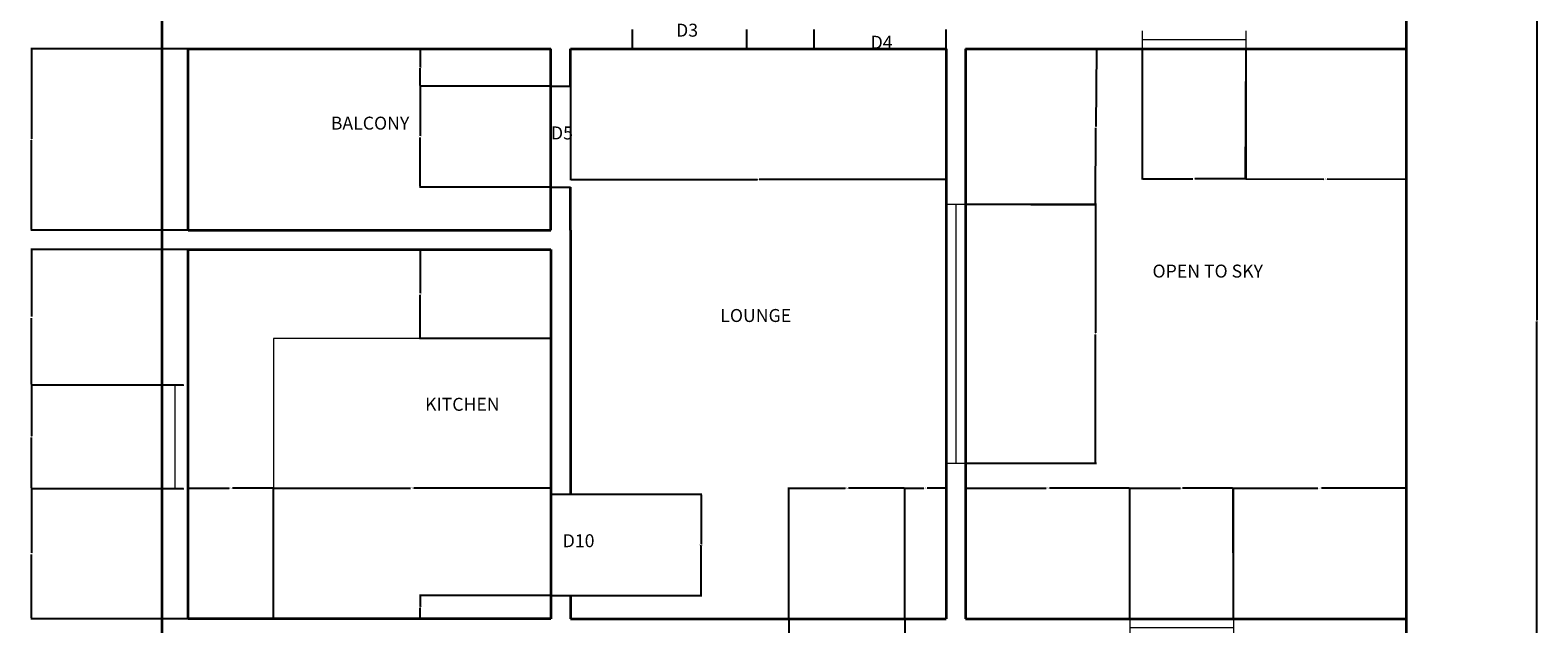
# Model space of a CAD drawing. Units: inches. Extents: x 301 to 1174, y -458 to 167.
# Tile 3 of 4: x 825 to 1174, y -203 to -66. Entities that reach past the tile are written whole.
import ezdxf

# ---------------------------------------------------------------- set-up
doc = ezdxf.new("R2010")
doc.units = ezdxf.units.IN
doc.header["$MEASUREMENT"] = 0
for name, color, linetype, lineweight in [('A-ANNO-DIMS', 2, 'Continuous', 18), ('A-ANNO-TEXT', 7, 'Continuous', 25), ('A-AREA-IDEN', 7, 'Continuous', 18), ('A-DOOR', 3, 'Continuous', 25), ('A-FLOR-FIXT', 8, 'Continuous', 18), ('A-GLAZ', 4, 'Continuous', 18), ('A-WALL', 7, 'Continuous', 35)]:
    doc.layers.add(name, color=color, linetype=linetype, lineweight=lineweight)
doc.styles.get("Standard").update_dxf_attribs({"font": 'arial.ttf'})
doc.dimstyles.get("Standard").update_dxf_attribs({"dimtxt": 0.18, "dimasz": 0.18, "dimexe": 0.18, "dimexo": 0.0625, "dimgap": 0.09, "dimtad": 0, "dimtih": 1, "dimtoh": 1, "dimdec": 4, "dimzin": 0, "dimdsep": 46, "dimtxsty": 'Standard', "dimcen": 0.09, "dimadec": 0, "dimazin": 0, "dimtfac": 1, "dimtdec": 4, "dimtofl": 0, "dimtmove": 0, "dimatfit": 3, "dimfxl": 1, "dimtolj": 1, "dimtzin": 0, "dimarcsym": 0})

# ---------------------------------------------------------------- blocks, each defined once
blk = doc.blocks.new('*U2')
for p, q in [((0, 4), (0, 0)), ((24, 4), (24, 0)), ((0, 2), (24, 2))]:
    blk.add_line(p, q)
blk = doc.blocks.new('*U4')
for p, q in [((0, 4), (0, 0)), ((60, 4), (60, 0)), ((0, 2), (60, 2))]:
    blk.add_line(p, q)
blk = doc.blocks.new('*D39')
at = {"layer": 'A-ANNO-DIMS', "color": 0, "lineweight": -2, "transparency": 16777216}
for p, q in [((1143.26, 136.8), (1173.63, 136.8)), ((1173.45, 136.62), (1173.45, -133.02)), ((1173.45, -403.02), (1173.45, -133.38)), ((1143.26, -403.2), (1173.63, -403.2))]:
    blk.add_line(p, q, dxfattribs=at)
at = {"layer": 'A-ANNO-DIMS', "color": 0, "transparency": 16777216}
for points in [[(1173.42, 136.62), (1173.48, 136.62), (1173.45, 136.8)], [(1173.42, -403.02), (1173.48, -403.02), (1173.45, -403.2)]]:
    blk.add_solid(points, dxfattribs=at)
at = {"layer": 'Defpoints', "color": 0, "transparency": 16777216}
for p in [(1143.2, 136.8), (1173.45, 136.8), (1143.2, -403.2)]:
    blk.add_point(p, dxfattribs=at)
at = {"layer": 'A-ANNO-DIMS', "color": 0, "transparency": 16777216, "insert": (1173.45, -133.2), "char_height": 0.18, "attachment_point": 5}
blk.add_mtext('\\A1;540', dxfattribs=at)
blk = doc.blocks.new('*D49')
at = {"layer": 'A-ANNO-DIMS', "color": 0, "lineweight": -2, "transparency": 16777216}
for p, q in [((861.2, -202.14), (861.2, -171.77)), ((861.38, -171.95), (870.71, -171.95)), ((880.81, -171.95), (871.48, -171.95)), ((880.99, -202.14), (880.99, -171.77))]:
    blk.add_line(p, q, dxfattribs=at)
at = {"layer": 'A-ANNO-DIMS', "color": 0, "transparency": 16777216}
for points in [[(861.38, -171.92), (861.38, -171.98), (861.2, -171.95)], [(880.81, -171.92), (880.81, -171.98), (880.99, -171.95)]]:
    blk.add_solid(points, dxfattribs=at)
at = {"layer": 'Defpoints', "color": 0, "transparency": 16777216}
for p in [(880.99, -171.95), (861.2, -202.2), (880.99, -202.2)]:
    blk.add_point(p, dxfattribs=at)
at = {"layer": 'A-ANNO-DIMS', "color": 0, "transparency": 16777216, "insert": (871.09, -171.95), "char_height": 0.18, "attachment_point": 5}
blk.add_mtext('\\A1;19.79', dxfattribs=at)
blk = doc.blocks.new('*D50')
at = {"layer": 'A-ANNO-DIMS', "color": 0, "lineweight": -2, "transparency": 16777216}
for p, q in [((880.99, -202.14), (880.99, -171.77)), ((881.17, -171.95), (912.72, -171.95)), ((945.02, -171.95), (913.47, -171.95)), ((945.2, -202.14), (945.2, -171.77))]:
    blk.add_line(p, q, dxfattribs=at)
at = {"layer": 'A-ANNO-DIMS', "color": 0, "transparency": 16777216}
for points in [[(881.17, -171.92), (881.17, -171.98), (880.99, -171.95)], [(945.02, -171.92), (945.02, -171.98), (945.2, -171.95)]]:
    blk.add_solid(points, dxfattribs=at)
at = {"layer": 'Defpoints', "color": 0, "transparency": 16777216}
for p in [(945.2, -171.95), (880.99, -202.2), (945.2, -202.2)]:
    blk.add_point(p, dxfattribs=at)
at = {"layer": 'A-ANNO-DIMS', "color": 0, "transparency": 16777216, "insert": (913.09, -171.95), "char_height": 0.18, "attachment_point": 5}
blk.add_mtext('\\A1;64.21', dxfattribs=at)
blk = doc.blocks.new('*D51')
at = {"layer": 'A-ANNO-DIMS', "color": 0, "lineweight": -2, "transparency": 16777216}
for p, q in [((945.13, -116.7), (914.77, -116.7)), ((914.95, -116.88), (914.95, -126.82)), ((914.95, -137.13), (914.95, -127.18)), ((945.13, -137.31), (914.77, -137.31))]:
    blk.add_line(p, q, dxfattribs=at)
at = {"layer": 'A-ANNO-DIMS', "color": 0, "transparency": 16777216}
for points in [[(914.92, -116.88), (914.98, -116.88), (914.95, -116.7)], [(914.92, -137.13), (914.98, -137.13), (914.95, -137.31)]]:
    blk.add_solid(points, dxfattribs=at)
at = {"layer": 'Defpoints', "color": 0, "transparency": 16777216}
for p in [(914.95, -116.7), (945.2, -116.7), (945.2, -137.31)]:
    blk.add_point(p, dxfattribs=at)
at = {"layer": 'A-ANNO-DIMS', "color": 0, "transparency": 16777216, "insert": (914.95, -127), "char_height": 0.18, "attachment_point": 5}
blk.add_mtext('\\A1;20.608', dxfattribs=at)
blk = doc.blocks.new('*D52')
at = {"layer": 'A-ANNO-DIMS', "color": 0, "lineweight": -2, "transparency": 16777216}
for p, q in [((949.7, -70.26), (949.7, -100.63)), ((1036.7, -70.26), (1036.7, -100.63)), ((949.88, -100.45), (992.98, -100.45)), ((1036.52, -100.45), (993.42, -100.45))]:
    blk.add_line(p, q, dxfattribs=at)
at = {"layer": 'A-ANNO-DIMS', "color": 0, "transparency": 16777216}
for points in [[(949.88, -100.42), (949.88, -100.48), (949.7, -100.45)], [(1036.52, -100.42), (1036.52, -100.48), (1036.7, -100.45)]]:
    blk.add_solid(points, dxfattribs=at)
at = {"layer": 'Defpoints', "color": 0, "transparency": 16777216}
for p in [(949.7, -70.2), (1036.7, -70.2), (949.7, -100.45)]:
    blk.add_point(p, dxfattribs=at)
at = {"layer": 'A-ANNO-DIMS', "color": 0, "transparency": 16777216, "insert": (993.2, -100.45), "char_height": 0.18, "attachment_point": 5}
blk.add_mtext('\\A1;87', dxfattribs=at)
blk = doc.blocks.new('*D59')
at = {"layer": 'A-ANNO-DIMS', "color": 0, "lineweight": -2, "transparency": 16777216}
for p, q in [((861.13, -70.2), (824.77, -70.2)), ((824.95, -70.38), (824.95, -91.02)), ((824.95, -112.02), (824.95, -91.38)), ((861.13, -112.2), (824.77, -112.2))]:
    blk.add_line(p, q, dxfattribs=at)
at = {"layer": 'A-ANNO-DIMS', "color": 0, "transparency": 16777216}
for points in [[(824.92, -70.38), (824.98, -70.38), (824.95, -70.2)], [(824.92, -112.02), (824.98, -112.02), (824.95, -112.2)]]:
    blk.add_solid(points, dxfattribs=at)
at = {"layer": 'Defpoints', "color": 0, "transparency": 16777216}
for p in [(824.95, -70.2), (861.2, -70.2), (861.2, -112.2)]:
    blk.add_point(p, dxfattribs=at)
at = {"layer": 'A-ANNO-DIMS', "color": 0, "transparency": 16777216, "insert": (824.95, -91.2), "char_height": 0.18, "attachment_point": 5}
blk.add_mtext('\\A1;42', dxfattribs=at)
blk = doc.blocks.new('*D60')
at = {"layer": 'A-ANNO-DIMS', "color": 0, "lineweight": -2, "transparency": 16777216}
for p, q in [((860.12, -172.08), (824.77, -172.08)), ((824.95, -172.26), (824.95, -186.96)), ((824.95, -202.02), (824.95, -187.32)), ((861.13, -202.2), (824.77, -202.2))]:
    blk.add_line(p, q, dxfattribs=at)
at = {"layer": 'A-ANNO-DIMS', "color": 0, "transparency": 16777216}
for points in [[(824.92, -172.26), (824.98, -172.26), (824.95, -172.08)], [(824.92, -202.02), (824.98, -202.02), (824.95, -202.2)]]:
    blk.add_solid(points, dxfattribs=at)
at = {"layer": 'Defpoints', "color": 0, "transparency": 16777216}
for p in [(824.95, -172.08), (860.18, -172.08), (861.2, -202.2)]:
    blk.add_point(p, dxfattribs=at)
at = {"layer": 'A-ANNO-DIMS', "color": 0, "transparency": 16777216, "insert": (824.95, -187.14), "char_height": 0.18, "attachment_point": 5}
blk.add_mtext('\\A1;30.12', dxfattribs=at)
blk = doc.blocks.new('*D61')
at = {"layer": 'A-ANNO-DIMS', "color": 0, "lineweight": -2, "transparency": 16777216}
for p, q in [((860.12, -148.08), (824.77, -148.08)), ((824.95, -148.26), (824.95, -159.9)), ((824.95, -171.9), (824.95, -160.26)), ((860.12, -172.08), (824.77, -172.08))]:
    blk.add_line(p, q, dxfattribs=at)
at = {"layer": 'A-ANNO-DIMS', "color": 0, "transparency": 16777216}
for points in [[(824.92, -148.26), (824.98, -148.26), (824.95, -148.08)], [(824.92, -171.9), (824.98, -171.9), (824.95, -172.08)]]:
    blk.add_solid(points, dxfattribs=at)
at = {"layer": 'Defpoints', "color": 0, "transparency": 16777216}
for p in [(824.95, -148.08), (860.18, -148.08), (860.18, -172.08)]:
    blk.add_point(p, dxfattribs=at)
at = {"layer": 'A-ANNO-DIMS', "color": 0, "transparency": 16777216, "insert": (824.95, -160.08), "char_height": 0.18, "attachment_point": 5}
blk.add_mtext('\\A1;24', dxfattribs=at)
blk = doc.blocks.new('*D62')
at = {"layer": 'A-ANNO-DIMS', "color": 0, "lineweight": -2, "transparency": 16777216}
for p, q in [((861.13, -116.7), (824.77, -116.7)), ((824.95, -116.88), (824.95, -132.21)), ((824.95, -147.9), (824.95, -132.57)), ((860.12, -148.08), (824.77, -148.08))]:
    blk.add_line(p, q, dxfattribs=at)
at = {"layer": 'A-ANNO-DIMS', "color": 0, "transparency": 16777216}
for points in [[(824.92, -116.88), (824.98, -116.88), (824.95, -116.7)], [(824.92, -147.9), (824.98, -147.9), (824.95, -148.08)]]:
    blk.add_solid(points, dxfattribs=at)
at = {"layer": 'Defpoints', "color": 0, "transparency": 16777216}
for p in [(824.95, -116.7), (861.2, -116.7), (860.18, -148.08)]:
    blk.add_point(p, dxfattribs=at)
at = {"layer": 'A-ANNO-DIMS', "color": 0, "transparency": 16777216, "insert": (824.95, -132.39), "char_height": 0.18, "attachment_point": 5}
blk.add_mtext('\\A1;31.38', dxfattribs=at)
blk = doc.blocks.new('*D78')
at = {"layer": 'A-ANNO-DIMS', "color": 0, "lineweight": -2, "transparency": 16777216}
for p, q in [((1082.02, -70.12), (1082.02, -100.48)), ((1106.02, -70.12), (1106.02, -100.48)), ((1082.2, -100.3), (1093.8, -100.3)), ((1105.84, -100.3), (1094.24, -100.3))]:
    blk.add_line(p, q, dxfattribs=at)
at = {"layer": 'A-ANNO-DIMS', "color": 0, "transparency": 16777216}
for points in [[(1082.2, -100.27), (1082.2, -100.33), (1082.02, -100.3)], [(1105.84, -100.27), (1105.84, -100.33), (1106.02, -100.3)]]:
    blk.add_solid(points, dxfattribs=at)
at = {"layer": 'Defpoints', "color": 0, "transparency": 16777216}
for p in [(1082.02, -70.05), (1106.02, -70.05), (1082.02, -100.3)]:
    blk.add_point(p, dxfattribs=at)
at = {"layer": 'A-ANNO-DIMS', "color": 0, "transparency": 16777216, "insert": (1094.02, -100.3), "char_height": 0.18, "attachment_point": 5}
blk.add_mtext('\\A1;24', dxfattribs=at)
blk = doc.blocks.new('*D79')
at = {"layer": 'A-ANNO-DIMS', "color": 0, "lineweight": -2, "transparency": 16777216}
for p, q in [((1106.02, -70.12), (1105.91, -100.48)), ((1143.2, -70.26), (1143.08, -100.63)), ((1106.09, -100.3), (1124.1, -100.37)), ((1142.9, -100.45), (1124.89, -100.38))]:
    blk.add_line(p, q, dxfattribs=at)
at = {"layer": 'A-ANNO-DIMS', "color": 0, "transparency": 16777216}
for points in [[(1106.09, -100.27), (1106.09, -100.33), (1105.91, -100.3)], [(1142.9, -100.42), (1142.9, -100.48), (1143.08, -100.45)]]:
    blk.add_solid(points, dxfattribs=at)
at = {"layer": 'Defpoints', "color": 0, "transparency": 16777216}
for p in [(1106.02, -70.05), (1143.2, -70.2), (1105.91, -100.3)]:
    blk.add_point(p, dxfattribs=at)
at = {"layer": 'A-ANNO-DIMS', "color": 0, "transparency": 16777216, "insert": (1124.49, -100.38), "char_height": 0.18, "attachment_point": 5}
blk.add_mtext('\\A1;37.17', dxfattribs=at)
blk = doc.blocks.new('*D80')
at = {"layer": 'A-ANNO-DIMS', "color": 0, "lineweight": -2, "transparency": 16777216}
for p, q in [((945.13, -78.86), (914.77, -78.86)), ((914.95, -79.04), (914.95, -90.36)), ((914.95, -102.04), (914.95, -90.72)), ((945.13, -102.22), (914.77, -102.22))]:
    blk.add_line(p, q, dxfattribs=at)
at = {"layer": 'A-ANNO-DIMS', "color": 0, "transparency": 16777216}
for points in [[(914.92, -79.04), (914.98, -79.04), (914.95, -78.86)], [(914.92, -102.04), (914.98, -102.04), (914.95, -102.22)]]:
    blk.add_solid(points, dxfattribs=at)
at = {"layer": 'Defpoints', "color": 0, "transparency": 16777216}
for p in [(914.95, -78.86), (945.2, -78.86), (945.2, -102.22)]:
    blk.add_point(p, dxfattribs=at)
at = {"layer": 'A-ANNO-DIMS', "color": 0, "transparency": 16777216, "insert": (914.95, -90.54), "char_height": 0.18, "attachment_point": 5}
blk.add_mtext('\\A1;23.355', dxfattribs=at)
blk = doc.blocks.new('*D81')
at = {"layer": 'A-ANNO-DIMS', "color": 0, "lineweight": -2, "transparency": 16777216}
for p, q in [((945.13, -70.2), (914.77, -70.2)), ((914.95, -70.38), (914.95, -74.35)), ((914.95, -78.68), (914.95, -74.71)), ((945.13, -78.86), (914.77, -78.86))]:
    blk.add_line(p, q, dxfattribs=at)
at = {"layer": 'A-ANNO-DIMS', "color": 0, "transparency": 16777216}
for points in [[(914.92, -70.38), (914.98, -70.38), (914.95, -70.2)], [(914.92, -78.68), (914.98, -78.68), (914.95, -78.86)]]:
    blk.add_solid(points, dxfattribs=at)
at = {"layer": 'Defpoints', "color": 0, "transparency": 16777216}
for p in [(914.95, -70.2), (945.2, -70.2), (945.2, -78.86)]:
    blk.add_point(p, dxfattribs=at)
at = {"layer": 'A-ANNO-DIMS', "color": 0, "transparency": 16777216, "insert": (914.95, -74.53), "char_height": 0.18, "attachment_point": 5}
blk.add_mtext('\\A1;8.662', dxfattribs=at)
blk = doc.blocks.new('*D82')
at = {"layer": 'A-ANNO-DIMS', "color": 0, "lineweight": -2, "transparency": 16777216}
for p, q in [((949.76, -173.33), (980.13, -173.33)), ((979.95, -173.51), (979.95, -184.91)), ((979.95, -196.67), (979.95, -185.27)), ((949.76, -196.85), (980.13, -196.85))]:
    blk.add_line(p, q, dxfattribs=at)
at = {"layer": 'A-ANNO-DIMS', "color": 0, "transparency": 16777216}
for points in [[(979.92, -173.51), (979.98, -173.51), (979.95, -173.33)], [(979.92, -196.67), (979.98, -196.67), (979.95, -196.85)]]:
    blk.add_solid(points, dxfattribs=at)
at = {"layer": 'Defpoints', "color": 0, "transparency": 16777216}
for p in [(949.7, -173.33), (949.7, -196.85), (979.95, -196.85)]:
    blk.add_point(p, dxfattribs=at)
at = {"layer": 'A-ANNO-DIMS', "color": 0, "transparency": 16777216, "insert": (979.95, -185.09), "char_height": 0.18, "attachment_point": 5}
blk.add_mtext('\\A1;23.523', dxfattribs=at)
blk = doc.blocks.new('*D83')
at = {"layer": 'A-ANNO-DIMS', "color": 0, "lineweight": -2, "transparency": 16777216}
for p, q in [((945.13, -196.85), (914.77, -196.85)), ((914.95, -197.03), (914.95, -199.34)), ((945.13, -202.2), (914.77, -202.2)), ((914.95, -202.02), (914.95, -199.71))]:
    blk.add_line(p, q, dxfattribs=at)
at = {"layer": 'A-ANNO-DIMS', "color": 0, "transparency": 16777216}
for points in [[(914.92, -197.03), (914.98, -197.03), (914.95, -196.85)], [(914.92, -202.02), (914.98, -202.02), (914.95, -202.2)]]:
    blk.add_solid(points, dxfattribs=at)
at = {"layer": 'Defpoints', "color": 0, "transparency": 16777216}
for p in [(914.95, -196.85), (945.2, -196.85), (945.2, -202.2)]:
    blk.add_point(p, dxfattribs=at)
at = {"layer": 'A-ANNO-DIMS', "color": 0, "transparency": 16777216, "insert": (914.95, -199.53), "char_height": 0.18, "attachment_point": 5}
blk.add_mtext('\\A1;5.347', dxfattribs=at)
blk = doc.blocks.new('*D84')
at = {"layer": 'A-ANNO-DIMS', "color": 0, "lineweight": -2, "transparency": 16777216}
for p, q in [((1041.26, -70.2), (1071.63, -70.34)), ((1071.45, -70.52), (1071.36, -88.16)), ((1071.28, -106.16), (1071.36, -88.52)), ((1041.09, -106.2), (1071.46, -106.34))]:
    blk.add_line(p, q, dxfattribs=at)
at = {"layer": 'A-ANNO-DIMS', "color": 0, "transparency": 16777216}
for points in [[(1071.42, -70.52), (1071.48, -70.52), (1071.45, -70.34)], [(1071.25, -106.16), (1071.31, -106.16), (1071.28, -106.34)]]:
    blk.add_solid(points, dxfattribs=at)
at = {"layer": 'Defpoints', "color": 0, "transparency": 16777216}
for p in [(1041.2, -70.2), (1041.03, -106.2), (1071.28, -106.34)]:
    blk.add_point(p, dxfattribs=at)
at = {"layer": 'A-ANNO-DIMS', "color": 0, "transparency": 16777216, "insert": (1071.36, -88.34), "char_height": 0.18, "attachment_point": 5}
blk.add_mtext('\\A1;36', dxfattribs=at)
blk = doc.blocks.new('*D85')
at = {"layer": 'A-ANNO-DIMS', "color": 0, "lineweight": -2, "transparency": 16777216}
for p, q in [((1041.09, -106.2), (1071.46, -106.2)), ((1071.28, -106.38), (1071.28, -136.02)), ((1071.28, -166.02), (1071.28, -136.38)), ((1041.09, -166.2), (1071.46, -166.2))]:
    blk.add_line(p, q, dxfattribs=at)
at = {"layer": 'A-ANNO-DIMS', "color": 0, "transparency": 16777216}
for points in [[(1071.25, -106.38), (1071.31, -106.38), (1071.28, -106.2)], [(1071.25, -166.02), (1071.31, -166.02), (1071.28, -166.2)]]:
    blk.add_solid(points, dxfattribs=at)
at = {"layer": 'Defpoints', "color": 0, "transparency": 16777216}
for p in [(1041.03, -106.2), (1041.03, -166.2), (1071.28, -166.2)]:
    blk.add_point(p, dxfattribs=at)
at = {"layer": 'A-ANNO-DIMS', "color": 0, "transparency": 16777216, "insert": (1071.28, -136.2), "char_height": 0.18, "attachment_point": 5}
blk.add_mtext('\\A1;60', dxfattribs=at)
blk = doc.blocks.new('*D86')
at = {"layer": 'A-ANNO-DIMS', "color": 0, "lineweight": -2, "transparency": 16777216}
for p, q in [((1000.23, -202.14), (1000.23, -171.77)), ((1000.41, -171.95), (1013.28, -171.95)), ((1026.93, -171.95), (1014.07, -171.95)), ((1027.11, -202.14), (1027.11, -171.77))]:
    blk.add_line(p, q, dxfattribs=at)
at = {"layer": 'A-ANNO-DIMS', "color": 0, "transparency": 16777216}
for points in [[(1000.41, -171.92), (1000.41, -171.98), (1000.23, -171.95)], [(1026.93, -171.92), (1026.93, -171.98), (1027.11, -171.95)]]:
    blk.add_solid(points, dxfattribs=at)
at = {"layer": 'Defpoints', "color": 0, "transparency": 16777216}
for p in [(1027.11, -171.95), (1000.23, -202.2), (1027.11, -202.2)]:
    blk.add_point(p, dxfattribs=at)
at = {"layer": 'A-ANNO-DIMS', "color": 0, "transparency": 16777216, "insert": (1013.67, -171.95), "char_height": 0.18, "attachment_point": 5}
blk.add_mtext('\\A1;26.88', dxfattribs=at)
blk = doc.blocks.new('*D87')
at = {"layer": 'A-ANNO-DIMS', "color": 0, "lineweight": -2, "transparency": 16777216}
for p, q in [((1027.11, -202.14), (1027.11, -171.77)), ((1027.29, -171.95), (1031.51, -171.95)), ((1036.52, -171.95), (1032.3, -171.95)), ((1036.7, -202.14), (1036.7, -171.77))]:
    blk.add_line(p, q, dxfattribs=at)
at = {"layer": 'A-ANNO-DIMS', "color": 0, "transparency": 16777216}
for points in [[(1027.29, -171.92), (1027.29, -171.98), (1027.11, -171.95)], [(1036.52, -171.92), (1036.52, -171.98), (1036.7, -171.95)]]:
    blk.add_solid(points, dxfattribs=at)
at = {"layer": 'Defpoints', "color": 0, "transparency": 16777216}
for p in [(1036.7, -171.95), (1027.11, -202.2), (1036.7, -202.2)]:
    blk.add_point(p, dxfattribs=at)
at = {"layer": 'A-ANNO-DIMS', "color": 0, "transparency": 16777216, "insert": (1031.9, -171.95), "char_height": 0.18, "attachment_point": 5}
blk.add_mtext('\\A1;9.585', dxfattribs=at)
blk = doc.blocks.new('*D88')
at = {"layer": 'A-ANNO-DIMS', "color": 0, "lineweight": -2, "transparency": 16777216}
for p, q in [((1041.2, -202.14), (1041.23, -171.77)), ((1041.41, -171.95), (1059.83, -171.97)), ((1079.03, -171.99), (1060.62, -171.97)), ((1079.18, -202.18), (1079.21, -171.81))]:
    blk.add_line(p, q, dxfattribs=at)
at = {"layer": 'A-ANNO-DIMS', "color": 0, "transparency": 16777216}
for points in [[(1041.41, -171.92), (1041.41, -171.98), (1041.23, -171.95)], [(1079.03, -171.96), (1079.03, -172.02), (1079.21, -171.99)]]:
    blk.add_solid(points, dxfattribs=at)
at = {"layer": 'Defpoints', "color": 0, "transparency": 16777216}
for p in [(1079.21, -171.99), (1041.2, -202.2), (1079.18, -202.24)]:
    blk.add_point(p, dxfattribs=at)
at = {"layer": 'A-ANNO-DIMS', "color": 0, "transparency": 16777216, "insert": (1060.22, -171.97), "char_height": 0.18, "attachment_point": 5}
blk.add_mtext('\\A1;37.98', dxfattribs=at)
blk = doc.blocks.new('*D89')
at = {"layer": 'A-ANNO-DIMS', "color": 0, "lineweight": -2, "transparency": 16777216}
for p, q in [((1079.18, -202.18), (1079.18, -171.81)), ((1079.36, -171.99), (1090.96, -171.99)), ((1103, -171.99), (1091.4, -171.99)), ((1103.18, -202.18), (1103.18, -171.81))]:
    blk.add_line(p, q, dxfattribs=at)
at = {"layer": 'A-ANNO-DIMS', "color": 0, "transparency": 16777216}
for points in [[(1079.36, -171.96), (1079.36, -172.02), (1079.18, -171.99)], [(1103, -171.96), (1103, -172.02), (1103.18, -171.99)]]:
    blk.add_solid(points, dxfattribs=at)
at = {"layer": 'Defpoints', "color": 0, "transparency": 16777216}
for p in [(1103.18, -171.99), (1079.18, -202.24), (1103.18, -202.24)]:
    blk.add_point(p, dxfattribs=at)
at = {"layer": 'A-ANNO-DIMS', "color": 0, "transparency": 16777216, "insert": (1091.18, -171.99), "char_height": 0.18, "attachment_point": 5}
blk.add_mtext('\\A1;24', dxfattribs=at)
blk = doc.blocks.new('*D90')
at = {"layer": 'A-ANNO-DIMS', "color": 0, "lineweight": -2, "transparency": 16777216}
for p, q in [((1103.18, -202.18), (1103.14, -171.81)), ((1103.32, -171.99), (1122.76, -171.97)), ((1142.98, -171.95), (1123.55, -171.97)), ((1143.2, -202.14), (1143.16, -171.77))]:
    blk.add_line(p, q, dxfattribs=at)
at = {"layer": 'A-ANNO-DIMS', "color": 0, "transparency": 16777216}
for points in [[(1103.32, -171.96), (1103.32, -172.02), (1103.14, -171.99)], [(1142.98, -171.92), (1142.98, -171.98), (1143.16, -171.95)]]:
    blk.add_solid(points, dxfattribs=at)
at = {"layer": 'Defpoints', "color": 0, "transparency": 16777216}
for p in [(1143.16, -171.95), (1103.18, -202.24), (1143.2, -202.2)]:
    blk.add_point(p, dxfattribs=at)
at = {"layer": 'A-ANNO-DIMS', "color": 0, "transparency": 16777216, "insert": (1123.15, -171.97), "char_height": 0.18, "attachment_point": 5}
blk.add_mtext('\\A1;40.02', dxfattribs=at)

msp = doc.modelspace()

# ---------------------------------------------------------------- linework, layer by layer
at = {"layer": 'A-DOOR'}
for p, q in [((963.9661, -65.6987), (963.9661, -70.1987)), ((990.4397, -65.6987), (990.4397, -70.1987)), ((1006.0166, -65.6987), (1006.0166, -70.1987)), ((1036.6974, -70.1987), (1036.6974, -65.6987)), ((945.1974, -78.8604), (949.6974, -78.8604)), ((945.1974, -102.2151), (949.6974, -102.2151)), ((945.1974, -173.3286), (949.6974, -173.3286)), ((945.1974, -196.8513), (949.6974, -196.8513)), ((1000.233, -202.1987), (1000.233, -206.6987)), ((1027.1125, -202.1987), (1027.1125, -206.6987))]:
    msp.add_line(p, q, dxfattribs=at)
at = {"layer": 'A-FLOR-FIXT'}
for p, q in [((945.1974, -137.3065), (880.9889, -137.3065)), ((880.9889, -137.3065), (880.9889, -202.1987)), ((945.1974, -137.3065), (945.1974, -137.3065))]:
    msp.add_line(p, q, dxfattribs=at)
at = {"layer": 'A-WALL'}
for p, q in [((855.1974, -403.1987), (855.1974, 136.8013)), ((1143.1974, 136.8013), (1143.1974, -403.1987)), ((861.1974, -112.1987), (861.1974, -70.1987)), ((861.1974, -70.1987), (945.1974, -70.1987)), ((945.1974, -112.1987), (945.1974, -70.1987)), ((949.6974, -70.1987), (996.1974, -70.1987)), ((949.6974, -78.8604), (949.6974, -70.1987)), ((996.1974, -70.1987), (1036.6974, -70.1987)), ((1036.6974, -70.1987), (1036.6974, -202.1987)), ((1041.1974, -70.1987), (1137.1974, -70.1987)), ((1041.1974, -70.1987), (1041.1974, -202.1987)), ((1137.1974, -70.1987), (1143.1974, -70.1987)), ((949.6974, -112.1987), (949.6974, -102.2151)), ((861.1974, -112.1987), (945.1974, -112.1987)), ((949.6974, -112.1987), (949.6974, -173.3286)), ((861.1974, -202.1987), (861.1974, -116.6987)), ((861.1974, -116.6987), (945.1974, -116.6987)), ((945.1974, -116.6987), (945.1974, -202.1987)), ((949.6974, -196.8513), (949.6974, -202.1987)), ((945.1974, -202.1987), (861.1974, -202.1987)), ((949.6974, -202.1987), (1036.6974, -202.1987)), ((1041.1974, -202.1987), (1137.1974, -202.1987)), ((1137.1974, -202.1987), (1143.1974, -202.1987))]:
    msp.add_line(p, q, dxfattribs=at)

# ---------------------------------------------------------------- block references
at = {"layer": 'A-GLAZ'}
for p in [(1082.0241, -70.0539), (1079.1778, -206.2439)]:
    msp.add_blockref('*U2', p, dxfattribs=at)
at = {"layer": 'A-GLAZ', "rotation": 90}
for name, p in [('*U4', (1041.03, -166.1987)), ('*U2', (860.1842, -172.0789))]:
    msp.add_blockref(name, p, dxfattribs=at)

# ---------------------------------------------------------------- texts
at = {"layer": 'A-ANNO-TEXT', "char_height": 3, "attachment_point": 1}
for s, insert in [('D3', (974.1661, -64.3886)), ('D4', (1019.2042, -67.1864)), ('D5', (945.1974, -88.1864)), ('D10', (947.921, -182.6295))]:
    msp.add_mtext_dynamic_manual_height_columns(s, width=13.351331, gutter_width=1, heights=[0], dxfattribs=dict(at, insert=insert))
at = {"layer": 'A-AREA-IDEN', "char_height": 0.2, "attachment_point": 1}
for s, insert in [('{\\H15x;BALCONY}', (894.2336, -85.9148)), ('{\\H15x;OPEN TO SKY}', (1084.4483, -120.1839)), ('{\\H15x;LOUNGE}', (984.4015, -130.4685)), ('{\\H15x;KITCHEN}', (916.0567, -151.0378))]:
    msp.add_mtext_dynamic_manual_height_columns(s, width=70.987625, gutter_width=1, heights=[0], dxfattribs=dict(at, insert=insert))

# ---------------------------------------------------------------- dimensions: what is measured, and where the dimension line sits
at = {"layer": 'A-ANNO-DIMS'}
for base, p1, p2, angle, override, picture, middle in [((1173.4474, 136.8013), (1143.1974, -403.1987), (1143.1974, 136.8013), 90, {"dimdec": 0, "dimlfac": 1, "dimrnd": 0, "dimzin": 0, "dimdsep": 46, "dimlunit": 2}, '*D39', (1173.4474, -133.1987)), ((824.9474, -70.1987), (861.1974, -112.1987), (861.1974, -70.1987), 90, {"dimdec": 0, "dimlfac": 1, "dimrnd": 0, "dimzin": 0, "dimdsep": 46, "dimlunit": 2}, '*D59', (824.9474, -91.1987)), ((914.9474, -70.1987), (945.1974, -78.8604), (945.1974, -70.1987), 90, {"dimdec": 3, "dimlfac": 1, "dimrnd": 0, "dimzin": 0, "dimdsep": 46, "dimlunit": 2}, '*D81', (914.9474, -74.5296)), ((949.6974, -100.4487), (1036.6974, -70.1987), (949.6974, -70.1987), 180, {"dimdec": 0, "dimlfac": 1, "dimrnd": 0, "dimzin": 0, "dimdsep": 46, "dimlunit": 2}, '*D52', (993.1974, -100.4487)), ((1071.2796, -106.3394), (1041.1974, -70.1987), (1041.03, -106.1987), 269.733465, {"dimdec": 0, "dimlfac": 1, "dimrnd": 0, "dimzin": 0, "dimdsep": 46, "dimlunit": 2}, '*D84', (1071.3634, -88.3394)), ((1082.0241, -100.3039), (1106.0241, -70.0539), (1082.0241, -70.0539), 180, {"dimdec": 0, "dimlfac": 1, "dimrnd": 0, "dimzin": 0, "dimdsep": 46, "dimlunit": 2}, '*D78', (1094.0241, -100.3039)), ((1105.9063, -100.3037), (1143.1974, -70.1987), (1106.0241, -70.0539), 179.776838, {"dimdec": 2, "dimlfac": 1, "dimrnd": 0, "dimzin": 0, "dimdsep": 46, "dimlunit": 2}, '*D79', (1124.493, -100.3761)), ((914.9474, -78.8604), (945.1974, -102.2151), (945.1974, -78.8604), 90, {"dimdec": 3, "dimlfac": 1, "dimrnd": 0, "dimzin": 0, "dimdsep": 46, "dimlunit": 2}, '*D80', (914.9474, -90.5378)), ((1071.28, -166.1987), (1041.03, -106.1987), (1041.03, -166.1987), 270, {"dimdec": 0, "dimlfac": 1, "dimrnd": 0, "dimzin": 0, "dimdsep": 46, "dimlunit": 2}, '*D85', (1071.28, -136.1987)), ((824.9474, -116.6987), (860.1842, -148.0789), (861.1974, -116.6987), 90, {"dimdec": 2, "dimlfac": 1, "dimrnd": 0, "dimzin": 0, "dimdsep": 46, "dimlunit": 2}, '*D62', (824.9474, -132.3888)), ((914.9474, -116.6987), (945.1974, -137.3065), (945.1974, -116.6987), 90, {"dimdec": 3, "dimlfac": 1, "dimrnd": 0, "dimzin": 0, "dimdsep": 46, "dimlunit": 2}, '*D51', (914.9474, -127.0026)), ((824.9474, -148.0789), (860.1842, -172.0789), (860.1842, -148.0789), 90, {"dimdec": 0, "dimlfac": 1, "dimrnd": 0, "dimzin": 0, "dimdsep": 46, "dimlunit": 2}, '*D61', (824.9474, -160.0789)), ((824.9474, -172.0789), (861.1974, -202.1987), (860.1842, -172.0789), 90, {"dimdec": 2, "dimlfac": 1, "dimrnd": 0, "dimzin": 0, "dimdsep": 46, "dimlunit": 2}, '*D60', (824.9474, -187.1388)), ((945.1974, -171.9487), (880.9889, -202.1987), (945.1974, -202.1987), 0, {"dimdec": 2, "dimlfac": 1, "dimrnd": 0, "dimzin": 0, "dimdsep": 46, "dimlunit": 2}, '*D50', (913.0932, -171.9487)), ((979.9474, -196.8513), (949.6974, -173.3286), (949.6974, -196.8513), 270, {"dimdec": 3, "dimlfac": 1, "dimrnd": 0, "dimzin": 0, "dimdsep": 46, "dimlunit": 2}, '*D82', (979.9474, -185.09)), ((1027.1125, -171.9487), (1000.233, -202.1987), (1027.1125, -202.1987), 0, {"dimdec": 2, "dimlfac": 1, "dimrnd": 0, "dimzin": 0, "dimdsep": 46, "dimlunit": 2}, '*D86', (1013.6727, -171.9487)), ((1079.2138, -171.9939), (1041.1974, -202.1987), (1079.1778, -202.2439), 359.931816, {"dimdec": 2, "dimlfac": 1, "dimrnd": 0, "dimzin": 0, "dimdsep": 46, "dimlunit": 2}, '*D88', (1060.2236, -171.9713)), ((1143.1633, -171.9487), (1103.1778, -202.2439), (1143.1974, -202.1987), 0.06471, {"dimdec": 2, "dimlfac": 1, "dimrnd": 0, "dimzin": 0, "dimdsep": 46, "dimlunit": 2}, '*D90', (1123.1535, -171.9713)), ((914.9474, -196.8513), (945.1974, -202.1987), (945.1974, -196.8513), 90, {"dimdec": 3, "dimlfac": 1, "dimrnd": 0, "dimzin": 0, "dimdsep": 46, "dimlunit": 2}, '*D83', (914.9474, -199.525))]:
    dim = msp.add_linear_dim(base=base, p1=p1, p2=p2, angle=angle, dimstyle='Standard', override=override, dxfattribs=at)
    dim.commit()
    dim.dimension.update_dxf_attribs({"geometry": picture, "text_midpoint": middle})
for base, p1, p2, override, picture, middle in [((880.9889, -171.9487), (861.1974, -202.1987), (880.9889, -202.1987), {"dimdec": 2, "dimlfac": 1, "dimrnd": 0, "dimzin": 0, "dimdsep": 46, "dimlunit": 2}, '*D49', (871.0932, -171.9487)), ((1036.6974, -171.9487), (1027.1125, -202.1987), (1036.6974, -202.1987), {"dimdec": 3, "dimlfac": 1, "dimrnd": 0, "dimzin": 0, "dimdsep": 46, "dimlunit": 2}, '*D87', (1031.905, -171.9487)), ((1103.1778, -171.9939), (1079.1778, -202.2439), (1103.1778, -202.2439), {"dimdec": 0, "dimlfac": 1, "dimrnd": 0, "dimzin": 0, "dimdsep": 46, "dimlunit": 2}, '*D89', (1091.1778, -171.9939))]:
    dim = msp.add_linear_dim(base=base, p1=p1, p2=p2, dimstyle='Standard', override=override, dxfattribs=at)
    dim.commit()
    dim.dimension.update_dxf_attribs({"geometry": picture, "text_midpoint": middle})

doc.saveas('drawing.dxf')
